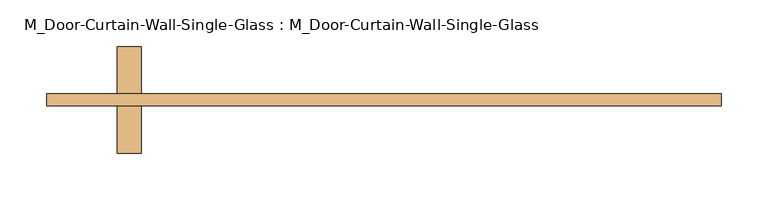
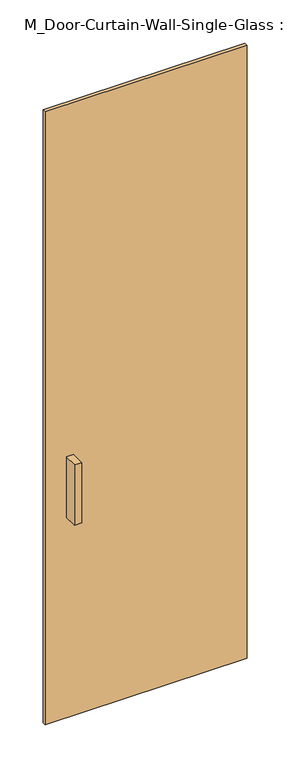
"""IFC4 building model written with IfcOpenShell, lengths in millimetres: door geometry, M_Door-Curtain-Wall-Single-Glass : M_Door-Curtain-Wall-Single-Glass."""

from ifc_helpers import new_model, si_unit, frame, origin, origin_with_axes, place, context, project, spatial, polyline, outline, extrude, source, transform, mapped, element, save


def m_door_curtain_wall_single_glass_m_door_curtain_wall_single_7bb093da(model_context):
    return source(origin(), model_context, "Body", "SweptSolid", [
        extrude(outline(polyline([(362.5, -50.8), (-362.5, -50.8), (-362.5, -38.1), (362.5, -38.1), (362.5, -50.8)])), origin_with_axes(), (0.0, 0.0, 1.0), 2325.0),
        extrude(outline(polyline([(-286.3, -101.6), (-286.3, -50.8), (-260.9, -50.8), (-260.9, -101.6), (-286.3, -101.6)])), frame((0.0, 0.0, 762.0), z_axis=(0.0, 0.0, 1.0), x_axis=(1.0, 0.0, 0.0)), (0.0, 0.0, 1.0), 228.6),
        extrude(outline(polyline([(-260.9, 12.7), (-260.9, -38.1), (-286.3, -38.1), (-286.3, 12.7), (-260.9, 12.7)])), frame((0.0, 0.0, 762.0), z_axis=(0.0, 0.0, 1.0), x_axis=(1.0, 0.0, 0.0)), (0.0, 0.0, 1.0), 228.6),
    ])


if __name__ == "__main__":
    model = new_model("IFC4")
    model_context = context("Model", 3, world=origin())
    ifc_project = project(units=[si_unit("LENGTHUNIT", "METRE", prefix="MILLI")], contexts=[model_context])
    site = spatial("IfcSite", under=ifc_project)
    building = spatial("IfcBuilding", under=site)
    placement = place(None, origin())
    m_door_curtain_wall_single_glass_m_door_curtain_wall_single_shape = m_door_curtain_wall_single_glass_m_door_curtain_wall_single_7bb093da(model_context)
    element("IfcDoor", 1, ObjectType="M_Door-Curtain-Wall-Single-Glass : M_Door-Curtain-Wall-Single-Glass", at=placement, inside=building, context=model_context, shape_type="MappedRepresentation", body=[
        mapped(m_door_curtain_wall_single_glass_m_door_curtain_wall_single_shape, transform((0.0, 0.0, 0.0), x_axis=(1.0, 0.0, 0.0), y_axis=(0.0, 1.0, 0.0), z_axis=(0.0, 0.0, 1.0))),
    ])
    save(model, "model.ifc")

# Revit data of these elements
# Type "M_Door-Curtain-Wall-Single-Glass : M_Door-Curtain-Wall-Single-Glass"
#   Type Mark = "46"
#   Assembly Code = "B2030100"
#   Analytic Construction = "<None>"
#   Width [instance default] = 900 mm
#   Thermal Resistance (R) = 1.7611 (m²·K)/W
#   Swing Angle [instance default] = 90.00°
#   Heat Transfer Coefficient (U) = 0.567826 W/(m²·K)
#   Offset = 50.8 mm
#   Define Thermal Properties by = 1
#   Function = 1
#   Door Handle Material = Aluminum
#   Glazing = Glass
#   Visual Light Transmittance = 0
#   Solar Heat Gain Coefficient = 0
#   Construction Type Id = ""
# Element 1 (IfcDoor, "M_Door-Curtain-Wall-Single-Glass : M_Door-Curtain-Wall-Single-Glass")
#   Width = 725 mm
#   Materials on its faces: "Aluminum", "Glass"
# Materials
#   "Aluminum": class "Metal", colour RGB 136 136 136, transparency 0, Description = "Aluminum 6061", Cost = 0
#   "Glass": class "Glass", colour RGB 245 245 243, transparency 1, Description = "Soda Lime Glass", Cost = 0
